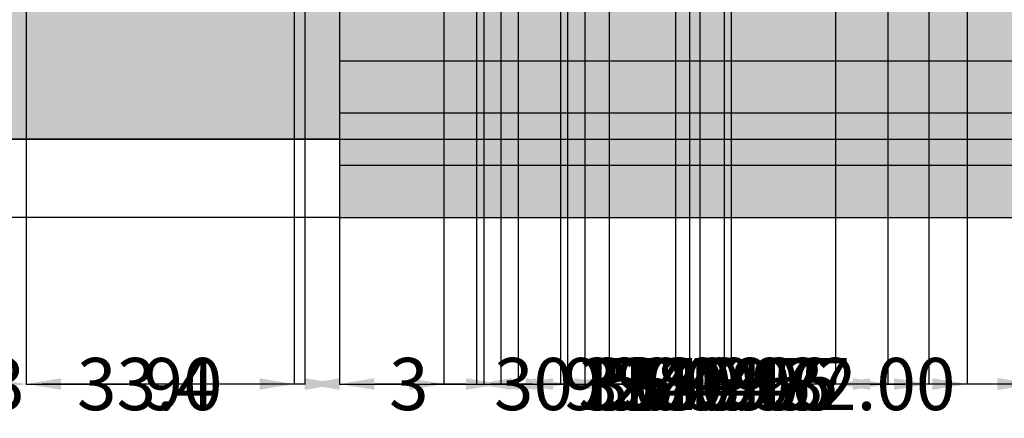
# Model space of a CAD drawing. Units: millimetres. Extents: x 131 to 845, y -20 to 1043.
# Tile 2 of 11: x 368 to 651, y -20 to 95. Entities that reach past the tile are written whole.
import ezdxf

# ---------------------------------------------------------------- set-up
doc = ezdxf.new("R2010")
doc.units = ezdxf.units.MM
doc.header["$MEASUREMENT"] = 0
for name, color, linetype, lineweight in [('A-ANNO-DIMS', 2, 'Continuous', 18), ('A-ELEV', 7, 'Continuous', 25), ('A-ELEV-PATT', 7, 'Continuous', 13), ('A-GLAZ-PATT', 143, 'Continuous', 13), ('A-WALL-PATT', 131, 'Continuous', 13)]:
    doc.layers.add(name, color=color, linetype=linetype, lineweight=lineweight)
doc.styles.get("Standard").update_dxf_attribs({"font": 'arial.ttf'})
doc.dimstyles.get("Standard").update_dxf_attribs({"dimtxt": 15, "dimasz": 10, "dimexe": 0.18, "dimexo": 0.0625, "dimgap": 5, "dimtad": 0, "dimtih": 1, "dimtoh": 1, "dimdec": 0, "dimzin": 0, "dimdsep": 46, "dimtxsty": 'Standard', "dimcen": 5, "dimadec": 0, "dimazin": 0, "dimtfac": 1, "dimtdec": 0, "dimtofl": 0, "dimtmove": 0, "dimatfit": 3, "dimfxl": 1, "dimtolj": 1, "dimtzin": 0, "dimarcsym": 0})

# ---------------------------------------------------------------- blocks, each defined once
blk = doc.blocks.new('*D14')
at = {"layer": 'A-ANNO-DIMS', "color": 0, "lineweight": -2, "transparency": 16777216}
for p, q in [((210.52, 985.67), (162.55, 985.67)), ((162.73, 975.67), (162.73, 524.4)), ((162.73, 47.81), (162.73, 499.08)), ((459.5, 37.81), (162.55, 37.81))]:
    blk.add_line(p, q, dxfattribs=at)
at = {"layer": 'A-ANNO-DIMS', "color": 0, "transparency": 16777216}
for points in [[(161.06, 975.67), (164.4, 975.67), (162.73, 985.67)], [(161.06, 47.81), (164.4, 47.81), (162.73, 37.81)]]:
    blk.add_solid(points, dxfattribs=at)
at = {"layer": 'Defpoints', "color": 0, "transparency": 16777216}
for p in [(162.73, 985.67), (210.58, 985.67), (459.56, 37.81)]:
    blk.add_point(p, dxfattribs=at)
at = {"layer": 'A-ANNO-DIMS', "color": 0, "transparency": 16777216, "insert": (162.73, 511.74), "char_height": 15, "attachment_point": 5}
blk.add_mtext('\\A1;947.9', dxfattribs=at)
blk = doc.blocks.new('*D18')
at = {"layer": 'A-ANNO-DIMS', "color": 0, "lineweight": -2, "transparency": 16777216}
for p, q in [((216.23, 60.25), (216.23, -10.22)), ((459.56, 60.25), (459.56, -10.22)), ((226.23, -10.04), (301.63, -10.04)), ((449.56, -10.04), (374.16, -10.04))]:
    blk.add_line(p, q, dxfattribs=at)
at = {"layer": 'A-ANNO-DIMS', "color": 0, "transparency": 16777216}
for points in [[(226.23, -8.37), (226.23, -11.7), (216.23, -10.04)], [(449.56, -8.37), (449.56, -11.7), (459.56, -10.04)]]:
    blk.add_solid(points, dxfattribs=at)
at = {"layer": 'Defpoints', "color": 0, "transparency": 16777216}
for p in [(216.23, 60.31), (459.56, 60.31), (459.56, -10.04)]:
    blk.add_point(p, dxfattribs=at)
at = {"layer": 'A-ANNO-DIMS', "color": 0, "transparency": 16777216, "insert": (337.9, -10.04), "char_height": 15, "attachment_point": 5}
blk.add_mtext('\\A1;243.33', dxfattribs=at)
blk = doc.blocks.new('*D33')
at = {"layer": 'A-ANNO-DIMS', "color": 0, "lineweight": -2, "transparency": 16777216}
for p, q in [((369.56, 283.49), (369.56, -10.22)), ((336.16, 178.37), (336.16, -10.22)), ((346.16, -10.04), (359.56, -10.04)), ((369.56, -10.04), (379.56, -10.04))]:
    blk.add_line(p, q, dxfattribs=at)
at = {"layer": 'A-ANNO-DIMS', "color": 0, "transparency": 16777216}
for points in [[(346.16, -8.37), (346.16, -11.7), (336.16, -10.04)], [(359.56, -8.37), (359.56, -11.7), (369.56, -10.04)]]:
    blk.add_solid(points, dxfattribs=at)
at = {"layer": 'Defpoints', "color": 0, "transparency": 16777216}
for p in [(369.56, 283.56), (336.16, 178.43), (369.56, -10.04)]:
    blk.add_point(p, dxfattribs=at)
at = {"layer": 'A-ANNO-DIMS', "color": 0, "transparency": 16777216, "insert": (404, -10.04), "char_height": 15, "attachment_point": 5}
blk.add_mtext('\\A1;33.4', dxfattribs=at)
blk = doc.blocks.new('*D34')
at = {"layer": 'A-ANNO-DIMS', "color": 0, "lineweight": -2, "transparency": 16777216}
for p, q in [((369.56, 283.49), (369.56, -10.22)), ((459.56, 283.49), (459.56, -10.22)), ((379.56, -10.04), (398.84, -10.04)), ((449.56, -10.04), (430.28, -10.04))]:
    blk.add_line(p, q, dxfattribs=at)
at = {"layer": 'A-ANNO-DIMS', "color": 0, "transparency": 16777216}
for points in [[(379.56, -8.37), (379.56, -11.7), (369.56, -10.04)], [(449.56, -8.37), (449.56, -11.7), (459.56, -10.04)]]:
    blk.add_solid(points, dxfattribs=at)
at = {"layer": 'Defpoints', "color": 0, "transparency": 16777216}
for p in [(369.56, 283.56), (459.56, 283.56), (459.56, -10.04)]:
    blk.add_point(p, dxfattribs=at)
at = {"layer": 'A-ANNO-DIMS', "color": 0, "transparency": 16777216, "insert": (414.56, -10.04), "char_height": 15, "attachment_point": 5}
blk.add_mtext('\\A1;90', dxfattribs=at)
blk = doc.blocks.new('*D37')
at = {"layer": 'A-ANNO-DIMS', "color": 0, "lineweight": -2, "transparency": 16777216}
for p, q in [((369.5, 283.56), (162.55, 283.56)), ((162.73, 273.56), (162.73, 184.6)), ((162.73, 70.31), (162.73, 159.27)), ((216.17, 60.31), (162.55, 60.31))]:
    blk.add_line(p, q, dxfattribs=at)
at = {"layer": 'A-ANNO-DIMS', "color": 0, "transparency": 16777216}
for points in [[(161.06, 273.56), (164.4, 273.56), (162.73, 283.56)], [(161.06, 70.31), (164.4, 70.31), (162.73, 60.31)]]:
    blk.add_solid(points, dxfattribs=at)
at = {"layer": 'Defpoints', "color": 0, "transparency": 16777216}
for p in [(369.56, 283.56), (162.73, 60.31), (216.23, 60.31)]:
    blk.add_point(p, dxfattribs=at)
at = {"layer": 'A-ANNO-DIMS', "color": 0, "transparency": 16777216, "insert": (162.73, 171.93), "char_height": 15, "attachment_point": 5}
blk.add_mtext('\\A1;223.24', dxfattribs=at)
blk = doc.blocks.new('*D50')
at = {"layer": 'A-ANNO-DIMS', "color": 0, "lineweight": -2, "transparency": 16777216}
for p, q in [((720.6, 488.6), (768.56, 488.6)), ((768.38, 478.6), (768.38, 287.12)), ((768.38, 70.31), (768.38, 261.79)), ((216.3, 60.31), (768.56, 60.31))]:
    blk.add_line(p, q, dxfattribs=at)
at = {"layer": 'A-ANNO-DIMS', "color": 0, "transparency": 16777216}
for points in [[(766.72, 478.6), (770.05, 478.6), (768.38, 488.6)], [(766.72, 70.31), (770.05, 70.31), (768.38, 60.31)]]:
    blk.add_solid(points, dxfattribs=at)
at = {"layer": 'Defpoints', "color": 0, "transparency": 16777216}
for p in [(720.53, 488.6), (768.38, 488.6), (216.23, 60.31)]:
    blk.add_point(p, dxfattribs=at)
at = {"layer": 'A-ANNO-DIMS', "color": 0, "transparency": 16777216, "insert": (768.38, 274.45), "char_height": 15, "attachment_point": 5}
blk.add_mtext('\\A1;428.3', dxfattribs=at)
blk = doc.blocks.new('*D51')
at = {"layer": 'A-ANNO-DIMS', "color": 0, "lineweight": -2, "transparency": 16777216}
for p, q in [((658.81, 488.53), (658.81, -10.22)), ((628.88, 312.6), (628.88, -10.22)), ((618.88, -10.04), (608.88, -10.04)), ((668.81, -10.04), (678.81, -10.04))]:
    blk.add_line(p, q, dxfattribs=at)
at = {"layer": 'A-ANNO-DIMS', "color": 0, "transparency": 16777216}
for points in [[(618.88, -8.37), (618.88, -11.7), (628.88, -10.04)], [(668.81, -8.37), (668.81, -11.7), (658.81, -10.04)]]:
    blk.add_solid(points, dxfattribs=at)
at = {"layer": 'Defpoints', "color": 0, "transparency": 16777216}
for p in [(658.81, 488.6), (628.88, 312.66), (658.81, -10.04)]:
    blk.add_point(p, dxfattribs=at)
at = {"layer": 'A-ANNO-DIMS', "color": 0, "transparency": 16777216, "insert": (715.07, -10.04), "char_height": 15, "attachment_point": 5}
blk.add_mtext('\\A1;29.923', dxfattribs=at)
blk = doc.blocks.new('*D52')
at = {"layer": 'A-ANNO-DIMS', "color": 0, "lineweight": -2, "transparency": 16777216}
for p, q in [((669.71, 488.53), (669.71, -10.22)), ((658.88, 312.6), (658.88, -10.22)), ((648.88, -10.04), (638.88, -10.04)), ((679.71, -10.04), (689.71, -10.04))]:
    blk.add_line(p, q, dxfattribs=at)
at = {"layer": 'A-ANNO-DIMS', "color": 0, "transparency": 16777216}
for points in [[(648.88, -8.37), (648.88, -11.7), (658.88, -10.04)], [(679.71, -8.37), (679.71, -11.7), (669.71, -10.04)]]:
    blk.add_solid(points, dxfattribs=at)
at = {"layer": 'Defpoints', "color": 0, "transparency": 16777216}
for p in [(669.71, 488.6), (658.88, 312.66), (669.71, -10.04)]:
    blk.add_point(p, dxfattribs=at)
at = {"layer": 'A-ANNO-DIMS', "color": 0, "transparency": 16777216, "insert": (725.2, -10.04), "char_height": 15, "attachment_point": 5}
blk.add_mtext('\\A1;10.825', dxfattribs=at)
blk = doc.blocks.new('*D62')
at = {"layer": 'A-ANNO-DIMS', "color": 0, "lineweight": -2, "transparency": 16777216}
for p, q in [((525.05, 459.74), (525.05, -10.22)), ((530.02, 454.68), (530.02, -10.22)), ((515.05, -10.04), (505.05, -10.04)), ((540.02, -10.04), (550.02, -10.04))]:
    blk.add_line(p, q, dxfattribs=at)
at = {"layer": 'A-ANNO-DIMS', "color": 0, "transparency": 16777216}
for points in [[(515.05, -8.37), (515.05, -11.7), (525.05, -10.04)], [(540.02, -8.37), (540.02, -11.7), (530.02, -10.04)]]:
    blk.add_solid(points, dxfattribs=at)
at = {"layer": 'Defpoints', "color": 0, "transparency": 16777216}
for p in [(525.05, 459.8), (530.02, 454.74), (530.02, -10.04)]:
    blk.add_point(p, dxfattribs=at)
at = {"layer": 'A-ANNO-DIMS', "color": 0, "transparency": 16777216, "insert": (580.63, -10.04), "char_height": 15, "attachment_point": 5}
blk.add_mtext('\\A1;4.977', dxfattribs=at)
blk = doc.blocks.new('*D65')
at = {"layer": 'A-ANNO-DIMS', "color": 0, "lineweight": -2, "transparency": 16777216}
for p, q in [((560.05, 439.74), (560.05, -10.22)), ((563.05, 439.74), (563.05, -10.22)), ((550.05, -10.04), (540.05, -10.04)), ((573.05, -10.04), (583.05, -10.04))]:
    blk.add_line(p, q, dxfattribs=at)
at = {"layer": 'A-ANNO-DIMS', "color": 0, "transparency": 16777216}
for points in [[(550.05, -8.37), (550.05, -11.7), (560.05, -10.04)], [(573.05, -8.37), (573.05, -11.7), (563.05, -10.04)]]:
    blk.add_solid(points, dxfattribs=at)
at = {"layer": 'Defpoints', "color": 0, "transparency": 16777216}
for p in [(560.05, 439.8), (563.05, 439.8), (563.05, -10.04)]:
    blk.add_point(p, dxfattribs=at)
at = {"layer": 'A-ANNO-DIMS', "color": 0, "transparency": 16777216, "insert": (592.96, -10.04), "char_height": 15, "attachment_point": 5}
blk.add_mtext('\\A1;3', dxfattribs=at)
blk = doc.blocks.new('*D67')
at = {"layer": 'A-ANNO-DIMS', "color": 0, "lineweight": -2, "transparency": 16777216}
for p, q in [((525.05, 459.74), (525.05, -10.22)), ((560.05, 439.74), (560.05, -10.22)), ((515.05, -10.04), (505.05, -10.04)), ((570.05, -10.04), (580.05, -10.04))]:
    blk.add_line(p, q, dxfattribs=at)
at = {"layer": 'A-ANNO-DIMS', "color": 0, "transparency": 16777216}
for points in [[(515.05, -8.37), (515.05, -11.7), (525.05, -10.04)], [(570.05, -8.37), (570.05, -11.7), (560.05, -10.04)]]:
    blk.add_solid(points, dxfattribs=at)
at = {"layer": 'Defpoints', "color": 0, "transparency": 16777216}
for p in [(525.05, 459.8), (560.05, 439.8), (560.05, -10.04)]:
    blk.add_point(p, dxfattribs=at)
at = {"layer": 'A-ANNO-DIMS', "color": 0, "transparency": 16777216, "insert": (542.55, -10.04), "char_height": 15, "attachment_point": 5}
blk.add_mtext('\\A1;35', dxfattribs=at)
blk = doc.blocks.new('*D68')
at = {"layer": 'A-ANNO-DIMS', "color": 0, "lineweight": -2, "transparency": 16777216}
for p, q in [((523.05, 305.1), (523.05, -10.22)), ((617.05, 305.1), (617.05, -10.22)), ((533.05, -10.04), (554.33, -10.04)), ((607.05, -10.04), (585.76, -10.04))]:
    blk.add_line(p, q, dxfattribs=at)
at = {"layer": 'A-ANNO-DIMS', "color": 0, "transparency": 16777216}
for points in [[(533.05, -8.37), (533.05, -11.7), (523.05, -10.04)], [(607.05, -8.37), (607.05, -11.7), (617.05, -10.04)]]:
    blk.add_solid(points, dxfattribs=at)
at = {"layer": 'Defpoints', "color": 0, "transparency": 16777216}
for p in [(523.05, 305.16), (617.05, 305.16), (617.05, -10.04)]:
    blk.add_point(p, dxfattribs=at)
at = {"layer": 'A-ANNO-DIMS', "color": 0, "transparency": 16777216, "insert": (570.05, -10.04), "char_height": 15, "attachment_point": 5}
blk.add_mtext('\\A1;94', dxfattribs=at)
blk = doc.blocks.new('*D69')
at = {"layer": 'A-ANNO-DIMS', "color": 0, "lineweight": -2, "transparency": 16777216}
for p, q in [((570.05, 303.56), (570.05, -10.22)), ((572.05, 303.56), (572.05, -10.22)), ((560.05, -10.04), (550.05, -10.04)), ((582.05, -10.04), (592.05, -10.04))]:
    blk.add_line(p, q, dxfattribs=at)
at = {"layer": 'A-ANNO-DIMS', "color": 0, "transparency": 16777216}
for points in [[(560.05, -8.37), (560.05, -11.7), (570.05, -10.04)], [(582.05, -8.37), (582.05, -11.7), (572.05, -10.04)]]:
    blk.add_solid(points, dxfattribs=at)
at = {"layer": 'Defpoints', "color": 0, "transparency": 16777216}
for p in [(570.05, 303.62), (572.05, 303.62), (572.05, -10.04)]:
    blk.add_point(p, dxfattribs=at)
at = {"layer": 'A-ANNO-DIMS', "color": 0, "transparency": 16777216, "insert": (616.63, -10.04), "char_height": 15, "attachment_point": 5}
blk.add_mtext('\\A1;2.00', dxfattribs=at)
blk = doc.blocks.new('*D70')
at = {"layer": 'A-ANNO-DIMS', "color": 0, "lineweight": -2, "transparency": 16777216}
for p, q in [((556.05, 309.1), (556.05, -10.22)), ((523.05, 305.1), (523.05, -10.22)), ((513.05, -10.04), (503.05, -10.04)), ((566.05, -10.04), (576.05, -10.04))]:
    blk.add_line(p, q, dxfattribs=at)
at = {"layer": 'A-ANNO-DIMS', "color": 0, "transparency": 16777216}
for points in [[(513.05, -8.37), (513.05, -11.7), (523.05, -10.04)], [(566.05, -8.37), (566.05, -11.7), (556.05, -10.04)]]:
    blk.add_solid(points, dxfattribs=at)
at = {"layer": 'Defpoints', "color": 0, "transparency": 16777216}
for p in [(556.05, 309.16), (523.05, 305.16), (556.05, -10.04)]:
    blk.add_point(p, dxfattribs=at)
at = {"layer": 'A-ANNO-DIMS', "color": 0, "transparency": 16777216, "insert": (539.55, -10.04), "char_height": 15, "attachment_point": 5}
blk.add_mtext('\\A1;33', dxfattribs=at)
blk = doc.blocks.new('*D71')
at = {"layer": 'A-ANNO-DIMS', "color": 0, "lineweight": -2, "transparency": 16777216}
for p, q in [((556.05, 309.1), (556.05, -10.22)), ((563.05, 309.1), (563.05, -10.22)), ((546.05, -10.04), (536.05, -10.04)), ((573.05, -10.04), (583.05, -10.04))]:
    blk.add_line(p, q, dxfattribs=at)
at = {"layer": 'A-ANNO-DIMS', "color": 0, "transparency": 16777216}
for points in [[(546.05, -8.37), (546.05, -11.7), (556.05, -10.04)], [(573.05, -8.37), (573.05, -11.7), (563.05, -10.04)]]:
    blk.add_solid(points, dxfattribs=at)
at = {"layer": 'Defpoints', "color": 0, "transparency": 16777216}
for p in [(556.05, 309.16), (563.05, 309.16), (563.05, -10.04)]:
    blk.add_point(p, dxfattribs=at)
at = {"layer": 'A-ANNO-DIMS', "color": 0, "transparency": 16777216, "insert": (592.9, -10.04), "char_height": 15, "attachment_point": 5}
blk.add_mtext('\\A1;7', dxfattribs=at)
blk = doc.blocks.new('*D72')
at = {"layer": 'A-ANNO-DIMS', "color": 0, "lineweight": -2, "transparency": 16777216}
for p, q in [((459.56, 300.1), (459.56, -10.22)), ((489.56, 300.1), (489.56, -10.22)), ((469.56, -10.04), (479.56, -10.04)), ((489.56, -10.04), (499.56, -10.04))]:
    blk.add_line(p, q, dxfattribs=at)
at = {"layer": 'A-ANNO-DIMS', "color": 0, "transparency": 16777216}
for points in [[(469.56, -8.37), (469.56, -11.7), (459.56, -10.04)], [(479.56, -8.37), (479.56, -11.7), (489.56, -10.04)]]:
    blk.add_solid(points, dxfattribs=at)
at = {"layer": 'Defpoints', "color": 0, "transparency": 16777216}
for p in [(459.56, 300.16), (489.56, 300.16), (489.56, -10.04)]:
    blk.add_point(p, dxfattribs=at)
at = {"layer": 'A-ANNO-DIMS', "color": 0, "transparency": 16777216, "insert": (515.27, -10.04), "char_height": 15, "attachment_point": 5}
blk.add_mtext('\\A1;30', dxfattribs=at)
blk = doc.blocks.new('*D79')
at = {"layer": 'A-ANNO-DIMS', "color": 0, "lineweight": -2, "transparency": 16777216}
for p, q in [((489.56, 300.1), (489.56, -10.22)), ((498.91, 291.72), (498.91, -10.22)), ((479.56, -10.04), (469.56, -10.04)), ((508.91, -10.04), (518.91, -10.04))]:
    blk.add_line(p, q, dxfattribs=at)
at = {"layer": 'A-ANNO-DIMS', "color": 0, "transparency": 16777216}
for points in [[(479.56, -8.37), (479.56, -11.7), (489.56, -10.04)], [(508.91, -8.37), (508.91, -11.7), (498.91, -10.04)]]:
    blk.add_solid(points, dxfattribs=at)
at = {"layer": 'Defpoints', "color": 0, "transparency": 16777216}
for p in [(489.56, 300.16), (498.91, 291.78), (498.91, -10.04)]:
    blk.add_point(p, dxfattribs=at)
at = {"layer": 'A-ANNO-DIMS', "color": 0, "transparency": 16777216, "insert": (549.23, -10.04), "char_height": 15, "attachment_point": 5}
blk.add_mtext('\\A1;9.349', dxfattribs=at)
blk = doc.blocks.new('*D80')
at = {"layer": 'A-ANNO-DIMS', "color": 0, "lineweight": -2, "transparency": 16777216}
for p, q in [((498.91, 291.72), (498.91, -10.22)), ((639.87, 291.72), (639.87, -10.22)), ((508.91, -10.04), (533.96, -10.04)), ((629.87, -10.04), (604.81, -10.04))]:
    blk.add_line(p, q, dxfattribs=at)
at = {"layer": 'A-ANNO-DIMS', "color": 0, "transparency": 16777216}
for points in [[(508.91, -8.37), (508.91, -11.7), (498.91, -10.04)], [(629.87, -8.37), (629.87, -11.7), (639.87, -10.04)]]:
    blk.add_solid(points, dxfattribs=at)
at = {"layer": 'Defpoints', "color": 0, "transparency": 16777216}
for p in [(498.91, 291.78), (639.87, 291.78), (639.87, -10.04)]:
    blk.add_point(p, dxfattribs=at)
at = {"layer": 'A-ANNO-DIMS', "color": 0, "transparency": 16777216, "insert": (569.39, -10.04), "char_height": 15, "attachment_point": 5}
blk.add_mtext('\\A1;140.96', dxfattribs=at)
blk = doc.blocks.new('*D82')
at = {"layer": 'A-ANNO-DIMS', "color": 0, "lineweight": -2, "transparency": 16777216}
for p, q in [((537.05, 283.2), (537.05, -10.22)), ((601.99, 283.2), (601.99, -10.22)), ((527.05, -10.04), (517.05, -10.04)), ((611.99, -10.04), (621.99, -10.04))]:
    blk.add_line(p, q, dxfattribs=at)
at = {"layer": 'A-ANNO-DIMS', "color": 0, "transparency": 16777216}
for points in [[(527.05, -8.37), (527.05, -11.7), (537.05, -10.04)], [(611.99, -8.37), (611.99, -11.7), (601.99, -10.04)]]:
    blk.add_solid(points, dxfattribs=at)
at = {"layer": 'Defpoints', "color": 0, "transparency": 16777216}
for p in [(537.05, 283.26), (601.99, 283.26), (601.99, -10.04)]:
    blk.add_point(p, dxfattribs=at)
at = {"layer": 'A-ANNO-DIMS', "color": 0, "transparency": 16777216, "insert": (569.52, -10.04), "char_height": 15, "attachment_point": 5}
blk.add_mtext('\\A1;64.95', dxfattribs=at)
blk = doc.blocks.new('*D84')
at = {"layer": 'A-ANNO-DIMS', "color": 0, "lineweight": -2, "transparency": 16777216}
for p, q in [((500.99, 289.46), (500.99, -10.22)), ((537.05, 283.2), (537.05, -10.22)), ((510.99, -10.04), (527.05, -10.04)), ((537.05, -10.04), (547.05, -10.04))]:
    blk.add_line(p, q, dxfattribs=at)
at = {"layer": 'A-ANNO-DIMS', "color": 0, "transparency": 16777216}
for points in [[(510.99, -8.37), (510.99, -11.7), (500.99, -10.04)], [(527.05, -8.37), (527.05, -11.7), (537.05, -10.04)]]:
    blk.add_solid(points, dxfattribs=at)
at = {"layer": 'Defpoints', "color": 0, "transparency": 16777216}
for p in [(500.99, 289.52), (537.05, 283.26), (537.05, -10.04)]:
    blk.add_point(p, dxfattribs=at)
at = {"layer": 'A-ANNO-DIMS', "color": 0, "transparency": 16777216, "insert": (577.41, -10.04), "char_height": 15, "attachment_point": 5}
blk.add_mtext('\\A1;36.05', dxfattribs=at)
blk = doc.blocks.new('*D86')
at = {"layer": 'A-ANNO-DIMS', "color": 0, "lineweight": -2, "transparency": 16777216}
for p, q in [((505.87, 97.75), (505.87, -10.22)), ((510.87, 97.75), (510.87, -10.22)), ((495.87, -10.04), (485.87, -10.04)), ((520.87, -10.04), (530.87, -10.04))]:
    blk.add_line(p, q, dxfattribs=at)
at = {"layer": 'A-ANNO-DIMS', "color": 0, "transparency": 16777216}
for points in [[(495.87, -8.37), (495.87, -11.7), (505.87, -10.04)], [(520.87, -8.37), (520.87, -11.7), (510.87, -10.04)]]:
    blk.add_solid(points, dxfattribs=at)
at = {"layer": 'Defpoints', "color": 0, "transparency": 16777216}
for p in [(505.87, 97.81), (510.87, 97.81), (510.87, -10.04)]:
    blk.add_point(p, dxfattribs=at)
at = {"layer": 'A-ANNO-DIMS', "color": 0, "transparency": 16777216, "insert": (540.84, -10.04), "char_height": 15, "attachment_point": 5}
blk.add_mtext('\\A1;5', dxfattribs=at)
blk = doc.blocks.new('*D91')
at = {"layer": 'A-ANNO-DIMS', "color": 0, "lineweight": -2, "transparency": 16777216}
for p, q in [((459.56, 37.75), (459.56, -10.22)), ((663.98, 37.75), (663.98, -10.22)), ((469.56, -10.04), (531.36, -10.04)), ((653.98, -10.04), (592.17, -10.04))]:
    blk.add_line(p, q, dxfattribs=at)
at = {"layer": 'A-ANNO-DIMS', "color": 0, "transparency": 16777216}
for points in [[(469.56, -8.37), (469.56, -11.7), (459.56, -10.04)], [(653.98, -8.37), (653.98, -11.7), (663.98, -10.04)]]:
    blk.add_solid(points, dxfattribs=at)
at = {"layer": 'Defpoints', "color": 0, "transparency": 16777216}
for p in [(459.56, 37.81), (663.98, 37.81), (663.98, -10.04)]:
    blk.add_point(p, dxfattribs=at)
at = {"layer": 'A-ANNO-DIMS', "color": 0, "transparency": 16777216, "insert": (561.77, -10.04), "char_height": 15, "attachment_point": 5}
blk.add_mtext('\\A1;204.4', dxfattribs=at)
blk = doc.blocks.new('*D92')
at = {"layer": 'A-ANNO-DIMS', "color": 0, "lineweight": -2, "transparency": 16777216}
for p, q in [((459.56, 67.75), (459.56, -10.22)), ((658.52, 67.75), (658.52, -10.22)), ((469.56, -10.04), (523.62, -10.04)), ((648.52, -10.04), (594.46, -10.04))]:
    blk.add_line(p, q, dxfattribs=at)
at = {"layer": 'A-ANNO-DIMS', "color": 0, "transparency": 16777216}
for points in [[(469.56, -8.37), (469.56, -11.7), (459.56, -10.04)], [(648.52, -8.37), (648.52, -11.7), (658.52, -10.04)]]:
    blk.add_solid(points, dxfattribs=at)
at = {"layer": 'Defpoints', "color": 0, "transparency": 16777216}
for p in [(459.56, 67.81), (658.52, 67.81), (658.52, -10.04)]:
    blk.add_point(p, dxfattribs=at)
at = {"layer": 'A-ANNO-DIMS', "color": 0, "transparency": 16777216, "insert": (559.04, -10.04), "char_height": 15, "attachment_point": 5}
blk.add_mtext('\\A1;198.96', dxfattribs=at)
blk = doc.blocks.new('*D99')
at = {"layer": 'A-ANNO-DIMS', "color": 0, "lineweight": -2, "transparency": 16777216}
for p, q in [((449.56, 833.53), (449.56, -10.22)), ((446.56, 818.53), (446.56, -10.22)), ((436.56, -10.04), (426.56, -10.04)), ((459.56, -10.04), (469.56, -10.04))]:
    blk.add_line(p, q, dxfattribs=at)
at = {"layer": 'A-ANNO-DIMS', "color": 0, "transparency": 16777216}
for points in [[(436.56, -8.37), (436.56, -11.7), (446.56, -10.04)], [(459.56, -8.37), (459.56, -11.7), (449.56, -10.04)]]:
    blk.add_solid(points, dxfattribs=at)
at = {"layer": 'Defpoints', "color": 0, "transparency": 16777216}
for p in [(449.56, 833.6), (446.56, 818.6), (449.56, -10.04)]:
    blk.add_point(p, dxfattribs=at)
at = {"layer": 'A-ANNO-DIMS', "color": 0, "transparency": 16777216, "insert": (479.47, -10.04), "char_height": 15, "attachment_point": 5}
blk.add_mtext('\\A1;3', dxfattribs=at)

msp = doc.modelspace()

# ---------------------------------------------------------------- hatches: boundary and pattern name
at = {"layer": 'A-ELEV-PATT', "transparency": 33554681}
h = msp.add_hatch(color=256, dxfattribs=at)
h.set_gradient(color1=(255, 255, 255), color2=(199, 200, 202), name='INVSPHERICAL')
h.paths.add_polyline_path([(489.5586, 300.1596), (459.5586, 300.1596), (459.5586, 252.07), (459.5586, 97.8131), (489.5586, 97.8131)])
h.paths.add_polyline_path([(680.5349, 300.1596), (650.5349, 300.1596), (650.5349, 97.8131), (680.5349, 97.8131)])
h.paths.add_polyline_path([(658.5215, 82.8131), (459.5586, 82.8131), (459.5586, 67.8131), (658.5215, 67.8131)])
h.paths.add_polyline_path([(663.9762, 52.8131), (459.5586, 52.8131), (459.5586, 37.8131), (663.9762, 37.8131)])
h.paths.add_polyline_path([(680.5349, 97.8131), (650.5349, 97.8131), (658.5215, 82.8131), (658.5215, 67.8131), (661.2489, 60.3131), (680.5349, 60.3131)])
at = {"layer": 'A-GLAZ-PATT'}
h = msp.add_hatch(color=256, dxfattribs=at)
h.dxf.hatch_style = 1
h.paths.add_polyline_path([(658.8074, 488.5953), (628.8842, 488.5953), (628.8842, 312.6596), (658.8842, 312.6596)])
h.paths.add_polyline_path([(650.5349, 97.8131), (459.5586, 97.8131), (459.5586, 82.8131), (658.5215, 82.8131)])
h.paths.add_polyline_path([(658.5215, 67.8131), (459.5586, 67.8131), (459.5586, 52.8131), (663.9762, 52.8131)])
at = {"layer": 'A-WALL-PATT'}
h = msp.add_hatch(color=256, dxfattribs=at)
h.dxf.hatch_style = 1
h.paths.add_polyline_path([(449.5586, 833.5953), (451.6297, 835.6663), (451.6297, 885.6663), (466.6297, 885.6663), (466.6297, 891.3345), (330.6595, 891.3345), (330.6595, 856.8345), (292.1595, 856.8345), (292.1595, 798.4332), (336.1595, 798.4332), (336.1595, 178.4332), (246.1595, 178.4332), (246.1595, 798.4332), (290.1595, 798.4332), (290.1595, 856.8345), (259.6595, 856.8345), (255.6595, 860.8345), (255.6595, 927.8345), (290.1595, 927.8345), (290.1595, 960.6663), (216.2327, 960.6663), (216.2327, 60.3131), (459.5586, 60.3131), (459.5586, 97.8131), (459.5586, 252.07), (459.5586, 283.5561), (369.5586, 283.5561), (369.5586, 763.5561), (439.5586, 763.5561), (439.5586, 778.6714), (439.5586, 793.5953), (439.5586, 796.5953), (441.5586, 798.5953), (444.5586, 798.5953), (444.5586, 813.5953), (444.5586, 816.5953), (446.5586, 818.5953), (449.5586, 818.5953)])
h.paths.add_polyline_path([(466.6297, 960.6663), (292.1595, 960.6663), (292.1595, 927.8345), (326.6595, 927.8345), (330.6595, 923.8345), (330.6595, 893.3345), (466.6297, 893.3345)], flags=17)
h.paths.add_polyline_path([(720.5349, 813.5953), (720.5349, 818.5953), (710.5349, 818.5953), (449.5586, 818.5953), (446.5586, 818.5953), (444.5586, 816.5953), (444.5586, 813.5953), (444.5586, 798.5953), (705.5349, 798.5953), (705.5349, 513.5953), (705.5349, 498.5953), (680.5349, 498.5953), (680.5349, 488.5953), (705.5349, 488.5953), (720.5349, 488.5953), (720.5349, 513.5953)])
h.paths.add_polyline_path([(680.5349, 498.5953), (412.6606, 498.5953), (412.6606, 488.5953), (680.5349, 488.5953)])

# ---------------------------------------------------------------- linework, layer by layer
at = {"layer": 'A-ELEV'}
for p, q in [((459.5586, 97.8131), (459.5586, 37.8131)), ((459.5586, 82.8131), (658.5215, 82.8131)), ((459.5586, 67.8131), (658.5215, 67.8131)), ((459.5586, 60.3131), (216.2327, 60.3131)), ((459.5586, 52.8131), (663.9762, 52.8131)), ((459.5586, 37.8131), (663.9762, 37.8131))]:
    msp.add_line(p, q, dxfattribs=at)

# ---------------------------------------------------------------- dimensions: what is measured, and where the dimension line sits
at = {"layer": 'A-ANNO-DIMS'}
for base, p1, p2, override, picture, middle in [((162.7317, 985.6663), (459.5586, 37.8131), (210.5817, 985.6663), {"dimdec": 1, "dimlfac": 1, "dimrnd": 0, "dimzin": 0, "dimdsep": 46, "dimlunit": 2}, '*D14', (162.7317, 511.7397)), ((768.3849, 488.5953), (216.2327, 60.3131), (720.5349, 488.5953), {"dimdec": 1, "dimlfac": 1, "dimrnd": 0, "dimzin": 0, "dimdsep": 46, "dimlunit": 2}, '*D50', (768.3849, 274.4542)), ((162.7317, 60.3131), (369.5586, 283.5561), (216.2327, 60.3131), {"dimdec": 2, "dimlfac": 1, "dimrnd": 0, "dimzin": 0, "dimdsep": 46, "dimlunit": 2}, '*D37', (162.7317, 171.9346))]:
    dim = msp.add_linear_dim(base=base, p1=p1, p2=p2, angle=90, dimstyle='Standard', override=override, dxfattribs=at)
    dim.commit()
    dim.dimension.update_dxf_attribs({"geometry": picture, "text_midpoint": middle})
for base, p1, p2, override, picture, middle in [((449.5586, -10.0369), (446.5586, 818.5953), (449.5586, 833.5953), {"dimdec": 0, "dimlfac": 1, "dimrnd": 0, "dimzin": 0, "dimdsep": 46, "dimlunit": 2}, '*D99', (479.4699, -10.0369)), ((658.8074, -10.0369), (628.8842, 312.6596), (658.8074, 488.5953), {"dimdec": 3, "dimlfac": 1, "dimrnd": 0, "dimzin": 0, "dimdsep": 46, "dimlunit": 2}, '*D51', (715.0711, -10.0369)), ((669.7096, -10.0369), (658.8842, 312.6596), (669.7096, 488.5953), {"dimdec": 3, "dimlfac": 1, "dimrnd": 0, "dimzin": 0, "dimdsep": 46, "dimlunit": 2}, '*D52', (725.1956, -10.0369)), ((530.0241, -10.0369), (525.0467, 459.8046), (530.0241, 454.7401), {"dimdec": 3, "dimlfac": 1, "dimrnd": 0, "dimzin": 0, "dimdsep": 46, "dimlunit": 2}, '*D62', (580.6346, -10.0369)), ((560.0467, -10.0369), (525.0467, 459.8046), (560.0467, 439.8046), {"dimdec": 0, "dimlfac": 1, "dimrnd": 0, "dimzin": 0, "dimdsep": 46, "dimlunit": 2}, '*D67', (542.5467, -10.0369)), ((563.0467, -10.0369), (560.0467, 439.8046), (563.0467, 439.8046), {"dimdec": 0, "dimlfac": 1, "dimrnd": 0, "dimzin": 0, "dimdsep": 46, "dimlunit": 2}, '*D65', (592.9581, -10.0369)), ((556.0467, -10.0369), (523.0467, 305.1596), (556.0467, 309.1596), {"dimdec": 0, "dimlfac": 1, "dimrnd": 0, "dimzin": 0, "dimdsep": 46, "dimlunit": 2}, '*D70', (539.5467, -10.0369)), ((563.0467, -10.0369), (556.0467, 309.1596), (563.0467, 309.1596), {"dimdec": 0, "dimlfac": 1, "dimrnd": 0, "dimzin": 0, "dimdsep": 46, "dimlunit": 2}, '*D71', (592.9018, -10.0369)), ((617.0467, -10.0369), (523.0467, 305.1596), (617.0467, 305.1596), {"dimdec": 0, "dimlfac": 1, "dimrnd": 0, "dimzin": 0, "dimdsep": 46, "dimlunit": 2}, '*D68', (570.0467, -10.0369)), ((572.0453, -10.0369), (570.0467, 303.6234), (572.0453, 303.6234), {"dimdec": 2, "dimlfac": 1, "dimrnd": 0, "dimzin": 0, "dimdsep": 46, "dimlunit": 2}, '*D69', (616.6292, -10.0369)), ((489.5586, -10.0369), (459.5586, 300.1596), (489.5586, 300.1596), {"dimdec": 0, "dimlfac": 1, "dimrnd": 0, "dimzin": 0, "dimdsep": 46, "dimlunit": 2}, '*D72', (515.2714, -10.0369)), ((498.9074, -10.0369), (489.5586, 300.1596), (498.9074, 291.7824), {"dimdec": 3, "dimlfac": 1, "dimrnd": 0, "dimzin": 0, "dimdsep": 46, "dimlunit": 2}, '*D79', (549.2314, -10.0369)), ((639.8713, -10.0369), (498.9074, 291.7824), (639.8713, 291.7824), {"dimdec": 2, "dimlfac": 1, "dimrnd": 0, "dimzin": 0, "dimdsep": 46, "dimlunit": 2}, '*D80', (569.3893, -10.0369)), ((537.0455, -10.0369), (500.9938, 289.5229), (537.0455, 283.2603), {"dimdec": 2, "dimlfac": 1, "dimrnd": 0, "dimzin": 0, "dimdsep": 46, "dimlunit": 2}, '*D84', (577.4053, -10.0369)), ((369.5586, -10.0369), (336.1595, 178.4332), (369.5586, 283.5561), {"dimdec": 1, "dimlfac": 1, "dimrnd": 0, "dimzin": 0, "dimdsep": 46, "dimlunit": 2}, '*D33', (404.0044, -10.0369)), ((459.5586, -10.0369), (369.5586, 283.5561), (459.5586, 283.5561), {"dimdec": 0, "dimlfac": 1, "dimrnd": 0, "dimzin": 0, "dimdsep": 46, "dimlunit": 2}, '*D34', (414.5586, -10.0369)), ((601.9946, -10.0369), (537.0455, 283.2603), (601.9946, 283.2603), {"dimdec": 2, "dimlfac": 1, "dimrnd": 0, "dimzin": 0, "dimdsep": 46, "dimlunit": 2}, '*D82', (569.5201, -10.0369)), ((510.8699, -10.0369), (505.8699, 97.8131), (510.8699, 97.8131), {"dimdec": 0, "dimlfac": 1, "dimrnd": 0, "dimzin": 0, "dimdsep": 46, "dimlunit": 2}, '*D86', (540.8426, -10.0369)), ((658.5215, -10.0369), (459.5586, 67.8131), (658.5215, 67.8131), {"dimdec": 2, "dimlfac": 1, "dimrnd": 0, "dimzin": 0, "dimdsep": 46, "dimlunit": 2}, '*D92', (559.0401, -10.0369)), ((459.5586, -10.0369), (216.2327, 60.3131), (459.5586, 60.3131), {"dimdec": 2, "dimlfac": 1, "dimrnd": 0, "dimzin": 0, "dimdsep": 46, "dimlunit": 2}, '*D18', (337.8956, -10.0369)), ((663.9762, -10.0369), (459.5586, 37.8131), (663.9762, 37.8131), {"dimdec": 1, "dimlfac": 1, "dimrnd": 0, "dimzin": 0, "dimdsep": 46, "dimlunit": 2}, '*D91', (561.7674, -10.0369))]:
    dim = msp.add_linear_dim(base=base, p1=p1, p2=p2, dimstyle='Standard', override=override, dxfattribs=at)
    dim.commit()
    dim.dimension.update_dxf_attribs({"geometry": picture, "text_midpoint": middle})

doc.saveas('drawing.dxf')
